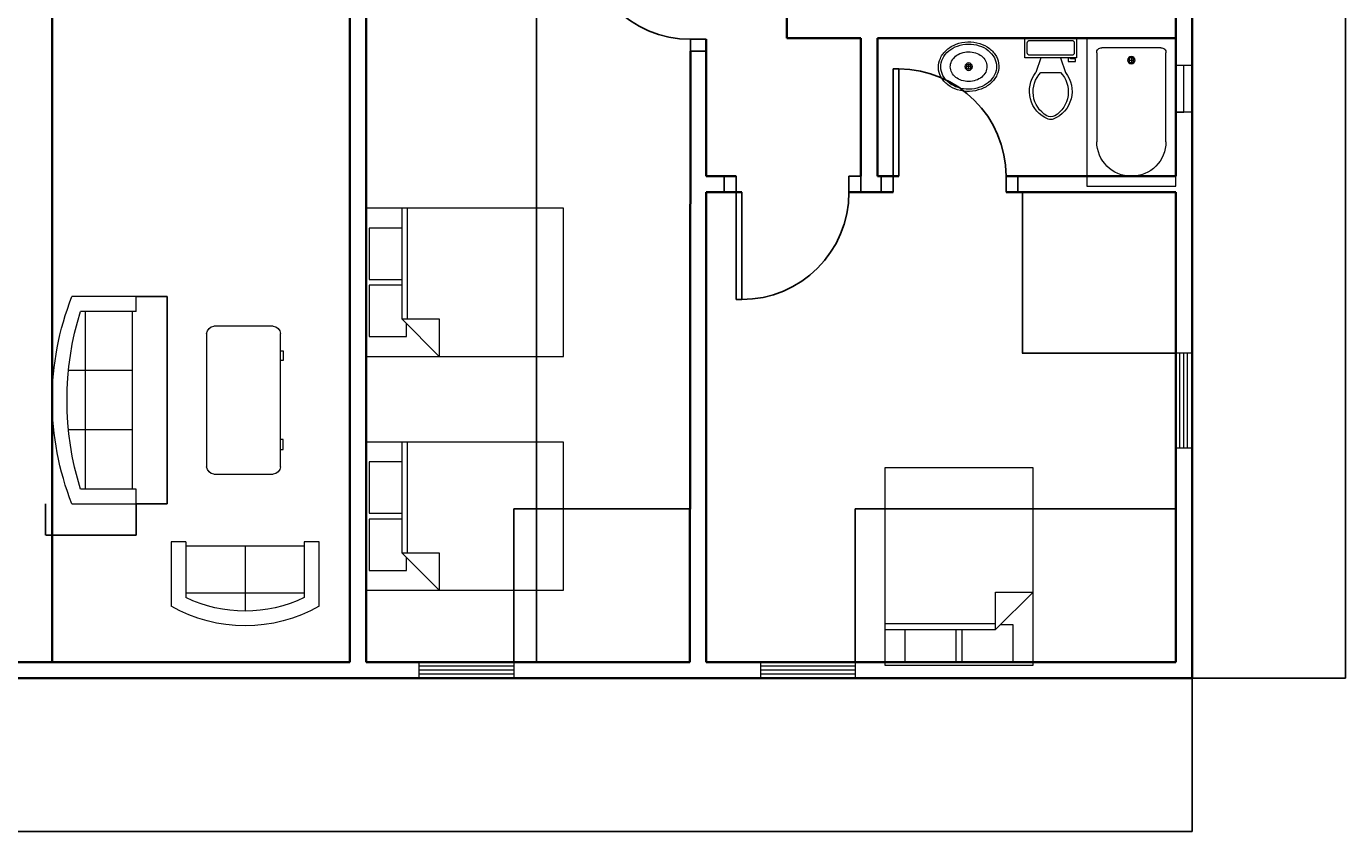
# Model space of a CAD drawing. Units: millimetres. Extents: x 31 to 27050, y -916 to 32407.
# Tile 4 of 7: x 13474 to 27050, y -916 to 7370. Entities that reach past the tile are written whole.
import ezdxf

# ---------------------------------------------------------------- set-up
doc = ezdxf.new("R2010")
doc.units = ezdxf.units.MM
for name, color, linetype, lineweight in [('A-ANNO-DIMS', 2, 'Continuous', 18), ('A-DOOR', 3, 'Continuous', 25), ('A-FLOR-FIXT', 9, 'Continuous', 18), ('A-FURN', 8, 'Continuous', 13), ('A-GLAZ', 4, 'Continuous', 18), ('A-WALL', 7, 'Continuous', 35)]:
    doc.layers.add(name, color=color, linetype=linetype, lineweight=lineweight)
doc.styles.get("Standard").update_dxf_attribs({"font": 'arial.ttf'})
doc.dimstyles.get("Standard").update_dxf_attribs({"dimtxt": 0.18, "dimasz": 0.18, "dimexe": 0.18, "dimexo": 0.0625, "dimgap": 0.09, "dimtad": 0, "dimtih": 1, "dimtoh": 1, "dimdec": 4, "dimzin": 0, "dimdsep": 46, "dimtxsty": 'Standard', "dimcen": 0.09, "dimadec": 0, "dimazin": 0, "dimtfac": 1, "dimtdec": 4, "dimtofl": 0, "dimtmove": 0, "dimatfit": 3, "dimfxl": 1, "dimtolj": 1, "dimtzin": 0, "dimarcsym": 0})

# ---------------------------------------------------------------- blocks, each defined once
blk = doc.blocks.new('Bath Tub - 26 x 60 in.')
for p, q in [((8, -18), (10, -18)), ((9, -17), (9, -19))]:
    blk.add_line(p, q)
blk.add_lwpolyline([(0, -36), (0, 0), (60, 0), (60, -36)], close=True)
for points in [[(6, -4), (42, -4)], [(4, -30), (4, -6)], [(42, -32), (6, -32)]]:
    blk.add_lwpolyline(points)
for radius in [1.5, 1]:
    blk.add_circle((9, -18), radius)
for centre, radius, start, end in [((5.75, -5.75), 1.767766999999999, 81.86989999999999, 188.1301), ((42, -18), 14, 270, 90), ((5.75, -30.25), 1.767766999999999, 171.8699, 278.1301)]:
    blk.add_arc(centre, radius, start, end)
blk = doc.blocks.new('Sink - Oval top')
for p, q in [((-1, 0), (1, 0)), ((0, 1), (0, -1))]:
    blk.add_line(p, q)
for points in [[(-12.23371880354079, 0.3941914712607968, 0.1176342565883263), (-11.46456229543957, -3.361933235489118, 0.104469279667093), (-8.878748691070427, -6.803541973650567, 0.0900157896014849), (-5.082757700676665, -9.072309807490512, 0.0819199491592185), (-0.3227280122732736, -10.01585280257211, 0.0819199491592091), (4.488169920880977, -9.380701564817912, 0.0900157896014801), (8.422342359155778, -7.36101289847943, 0.1044692796670922), (11.22435122606941, -4.093009071543406, 0.1176342565883338), (12.23371880354091, -0.3941914712607968, 0.1176342565883057), (11.46456229543992, 3.361933235488777, 0.1044692796670849), (8.878748691070427, 6.803541973650567, 0.0900157896014884), (5.082757700676324, 9.072309807490681, 0.0819199491592058), (0.3227280122732736, 10.01585280257211, 0.081919949159207), (-4.488169920880864, 9.380701564817969, 0.0900157896014802), (-8.422342359155778, 7.36101289847943, 0.1044692796670951), (-11.22435122606919, 4.093009071543633, 0.1176342565883402)], [(-11.28627986850119, 0.1590597164737346, 0.1186217001864142), (-10.51590095791209, -3.253161772358112, 0.1046781721811095), (-8.071803350560115, -6.358618019863342, 0.0895620664691738), (-4.537699193222351, -8.366971929609804, 0.0811846988912177), (-0.1289739026695997, -9.15150355811437, 0.0811846988912276), (4.300109150126218, -8.491524865184601, 0.0895620664691798), (7.889406708212618, -6.583562428127606, 0.1046781721811044), (10.42004782883111, -3.548216131892445, 0.1186217001864013), (11.28627986850119, -0.1590597164736209, 0.1186217001863945), (10.51590095791221, 3.253161772357998, 0.1046781721811069), (8.071803350560115, 6.358618019863342, 0.0895620664691756), (4.537699193222124, 8.366971929609917, 0.081184698891216), (0.1289739026695997, 9.151503558114428, 0.0811846988912142), (-4.300109150125877, 8.491524865184829, 0.0895620664691747), (-7.889406708212618, 6.583562428127606, 0.1046781721811045), (-10.42004782883111, 3.548216131892445, 0.1186217001863946)], [(-7.420452389032902, 0.0829876781601797, 0.1182825673856775), (-6.907065465214486, -2.1674649380775, 0.1046074595377274), (-5.294791470712084, -4.209988192029413, 0.0897179636260996), (-2.966599981142508, -5.528122152688069, 0.0814360825277113), (-0.0675135187855176, -6.036810076758797, 0.0814360825277218), (2.84222437824053, -5.593085960977873, 0.0897179636261315), (5.199312936802016, -4.327350491993342, 0.1046074595376878), (6.85686365682659, -2.321395784920355, 0.1182825673856714), (7.420452389033016, -0.0829876781601797, 0.1182825673856961), (6.907065465214486, 2.167464938077614, 0.1046074595377135), (5.294791470712084, 4.209988192029413, 0.0897179636261265), (2.966599981142621, 5.528122152687842, 0.0814360825277426), (0.0675135187855176, 6.036810076758797, 0.0814360825277225), (-2.842224378240644, 5.593085960977873, 0.0897179636261212), (-5.199312936802016, 4.327350491993342, 0.1046074595377049), (-6.856863656826476, 2.321395784920355, 0.1182825673856712)]]:
    blk.add_lwpolyline(points, format="xyb", close=True)
for radius in [1.5, 1]:
    blk.add_circle((0, 0), radius)
blk = doc.blocks.new('Toilet - top')
for p, q in [((9.5, -6), (9.5, -2)), ((-10, -8.5), (-8, -8.5)), ((-10, -9.5), (-10, -8.5)), ((-7, -9.5), (-10, -9.5)), ((-8, -8.5), (-8, -8)), ((-7, -8), (-7, -9.5)), ((-4, -8), (-6, -14)), ((4, -8), (6, -14)), ((4, -14), (-4, -14))]:
    blk.add_line(p, q)
blk.add_lwpolyline([(10.5, -8), (10.5, 0), (-10.5, 0), (-10.5, -8)], close=True)
for points in [[(-9.5, -2), (-9.5, -6)], [(8.5, -1), (-8.5, -1)], [(-8.5, -7), (8.5, -7)]]:
    blk.add_lwpolyline(points)
for centre, radius, start, end in [((-8.625, -1.875), 0.8838834999999999, 81.86989999999999, 188.1301), ((8.625, -1.875), 0.8838834999999999, 351.8699, 98.13009999999998), ((-8.625, -6.125), 0.8838834999999999, 171.869898, 278.1301), ((8.625, -6.125), 0.8838834999999999, 261.8699, 8.130099999999993), ((3.519562435188956, -21.58049502388982), 12.16902005083646, 141.4691096810948, 247.9714346835576), ((4.199957580658807, -21.81740929088453), 11.3291791325804, 136.3677254423718, 238.946823937405), ((-3.519499936778316, -21.58047137067522), 12.16903423757823, 292.0284332733152, 38.53070636800453), ((-4.199890672038477, -21.81738596564128), 11.32918622148567, 301.0530065773863, 43.63209216694732), ((2.09660981727e-05, -27.87646475467881), 4, 245.7318247449371, 294.2681740488959), ((2.09415214183e-05, -28.99996806116075), 4, 254.8605283244437, 285.1394707718433)]:
    blk.add_arc(centre, radius, start, end)
blk = doc.blocks.new('Sofa - Roundback 7 ft.')
for p, q in [((-12.00002, -32.44210000000393), (-12.00003, -6.597100000003898)), ((11.99996999999999, -32.44210000000393), (11.99997999999999, -6.597100000003898)), ((-36.000027, -34.00000000000395), (-36.000027, -11.46960000000396)), ((-35.999844, -13.38190000000397), (35.99979999999999, -13.38190000000397)), ((35.99997999999999, -34.00000000000395), (35.99997999999999, -11.46960000000396)), ((-36.000027, -32.44210000000393), (35.99997999999999, -32.44210000000393))]:
    blk.add_line(p, q)
for points in [[(-36.000027, -34.00000000000395), (-42.000027, -34.00000000000395), (-42.000027, -8.000000000003944)], [(41.99997999999999, -8.000000000003944), (41.99997999999999, -34.00000000000395), (35.99997999999999, -34.00000000000395)]]:
    blk.add_lwpolyline(points)
for centre, radius, start, end in [((0, -114.2500000000039), 114.2500000000039, 68.43141000000072, 111.5686000000006), ((-1.00000000032e-05, -127.1968000000039), 121.1967999999973, 72.72032999999948, 107.2797000000005)]:
    blk.add_arc(centre, radius, start, end)
blk = doc.blocks.new('Sofa - Roundback Loveseat 5 ft.')
for p, q in [((0, -32.44198000000246), (0, -5.999980000002448)), ((-23.99999999999999, -33.99998000000245), (-23.99999999999999, -11.46958000000243)), ((-23.99979999999998, -13.38178000000245), (23.99986, -13.38178000000245)), ((24.00004000000001, -33.99998000000245), (24.00004000000001, -11.46958000000243)), ((-23.99999999999999, -32.44198000000246), (24.00004000000001, -32.44198000000246))]:
    blk.add_line(p, q)
for points in [[(-23.99999999999999, -33.99998000000245), (-29.99999999999999, -33.99998000000245), (-29.99999999999999, -7.999980000002448)], [(30.00004000000001, -7.999980000002448), (30.00004000000001, -33.99998000000245), (24.00004000000001, -33.99998000000245)]]:
    blk.add_lwpolyline(points)
for centre, radius, start, end in [((0, -60.24998000000245), 60.24998000000245, 60.13715000000122, 119.862800000004), ((0, -61.38438000000245), 55.38444000000723, 64.32083000000306, 115.6791999999996)]:
    blk.add_arc(centre, radius, start, end)
blk = doc.blocks.new('Desk - 30 x 60 in.')
for p, q in [((-26.999995, 0), (26.999995, 0)), ((-29.999995, -27), (-29.999995, -3)), ((29.999995, -3), (29.999995, -27)), ((26.999995, -30), (-26.999995, -30)), ((-20.000005, -30), (-20.000005, -31)), ((-20.000005, -31), (-16.000005, -31)), ((-16.000005, -31), (-16.000005, -30)), ((15.999995, -31), (15.999995, -30)), ((19.999995, -31), (15.999995, -31)), ((19.999995, -30), (19.999995, -31))]:
    blk.add_line(p, q)
for centre, radius, start, end in [((-26.499995, -3.5), 3.535534000004229, 98.1300999999916, 171.8698999999352), ((26.499995, -3.5), 3.535533999997753, 8.130102000022115, 81.8698999999439), ((-26.499995, -26.5), 3.535534000000845, 188.1301000000653, 261.8699000000085), ((26.499995, -26.5), 3.535534000004826, 278.1301000000561, 351.8698999999439)]:
    blk.add_arc(centre, radius, start, end)
blk = doc.blocks.new('Bed - Queen')
for p, q in [((0, -80.00003000000002), (0, 0)), ((0, 0), (59.99998999999999, 0)), ((59.99998999999999, 0), (59.99998999999999, -80.00003000000002)), ((7.99999, -1.200000000000017), (28.79998, -1.200000000000017)), ((7.99999, -14.4), (7.99999, -1.200000000000017)), ((28.79998, -1.200000000000017), (28.79998, -14.4)), ((31.19999, -1.200000000000017), (51.99999000000001, -1.200000000000017)), ((31.19999, -14.4), (31.19999, -1.200000000000017)), ((51.99999000000001, -1.200000000000017), (51.99999000000001, -16.4)), ((0, -14.4), (44.79999999999999, -14.4)), ((59.99998999999999, -29.60000000000001), (44.79999999999999, -14.4)), ((44.79999999999999, -14.4), (44.79999999999999, -29.60000000000001)), ((44.79999999999999, -16.80000000000001), (0, -16.80000000000001)), ((51.99999000000001, -16.4), (46.79936, -16.4)), ((44.79999999999999, -29.60000000000001), (59.99998999999999, -29.60000000000001)), ((59.99998999999999, -80.00003000000002), (0, -80.00003000000002))]:
    blk.add_line(p, q)
blk = doc.blocks.new('Window - Wood Frame 36 in. Wide plan')
for p, q in [((0, 6), (0, 0)), ((36, 6), (36, 0)), ((0, 4.5), (36, 4.5)), ((0, 3), (36, 3)), ((0, 1.5), (36, 1.5))]:
    blk.add_line(p, q)
blk = doc.blocks.new('DOOR-SINGLE-1104')
for p, q in [((56.41678681898429, 1104.337341461596), (-7.18501e-11, 1104.337341461596)), ((-7.18501e-11, 1104.337341461596), (-7.18501e-11, 3.638e-12)), ((56.41678681898429, 7.276e-12), (56.41678681898429, 1104.337341461596)), ((-1226.913698425656, -163.8831223050438), (-1226.913698425656, 3.638e-12)), ((-1104.337341461589, 3.638e-12), (-1226.913698425656, 7.276e-12)), ((-1104.337341461589, 3.638e-12), (-1104.337341461589, -163.8831223050438)), ((-7.18501e-11, 3.638e-12), (56.41678681898429, 7.276e-12)), ((56.41678681898429, -163.8831223050438), (56.41678681898429, 3.638e-12)), ((56.41678681898429, 3.638e-12), (178.9931437830519, 3.638e-12)), ((178.9931437830519, 3.638e-12), (178.9931437830519, -163.8831223050438)), ((-1104.337341461589, -163.8831223050438), (-1226.913698425656, -163.8831223050438)), ((178.9931437830519, -163.8831223050438), (56.41678681898429, -163.8831223050438))]:
    blk.add_line(p, q)
blk.add_arc((0, 3.638e-12), 1104.337341461589, 90, 180)
blk = doc.blocks.new('WIN-BATH-482-FRAMED')
for p, q in [((-2.274e-13, -9.095e-13), (-168.3506507106942, -9.095e-13)), ((-168.3506507106942, -9.095e-13), (-168.3506507106942, -482.3297634273203)), ((-84.17532535534656, -482.3297634273203), (-84.17532535534723, -9.095e-13)), ((-168.3506507106942, -482.3297634273203), (1.1369e-12, -482.3297634273195)), ((1.1369e-12, -482.3297634273195), (-84.17532535534656, -482.3297634273203))]:
    blk.add_line(p, q)
blk = doc.blocks.new('*D34')
at = {"layer": 'A-ANNO-DIMS', "color": 0, "lineweight": -2, "transparency": 16777216}
for p, q in [((14604.24783261055, 4589.760747355135), (14924.40539496012, 4589.760747355135)), ((14924.22539496012, 4589.580747355134), (14924.22539496012, 3523.143731883442)), ((14924.22539496012, 2456.340331691422), (14924.22539496012, 3522.777347163115)), ((14604.24783261055, 2456.160331691423), (14924.40539496012, 2456.160331691423))]:
    blk.add_line(p, q, dxfattribs=at)
at = {"layer": 'A-ANNO-DIMS', "color": 0, "transparency": 16777216}
for points in [[(14924.19539496012, 4589.580747355134), (14924.25539496012, 4589.580747355134), (14924.22539496012, 4589.760747355135)], [(14924.19539496012, 2456.340331691422), (14924.25539496012, 2456.340331691422), (14924.22539496012, 2456.160331691423)]]:
    blk.add_solid(points, dxfattribs=at)
at = {"layer": 'Defpoints', "color": 0, "transparency": 16777216}
for p in [(14604.18533261055, 4589.760747355135), (14604.18533261055, 2456.160331691423), (14924.22539496012, 2456.160331691423)]:
    blk.add_point(p, dxfattribs=at)
at = {"layer": 'A-ANNO-DIMS', "color": 0, "transparency": 16777216, "insert": (14924.22539496011, 3522.960539523273), "char_height": 0.18, "attachment_point": 5}
blk.add_mtext('\\A1;SOFA 2134 TYP.', dxfattribs=at)
blk = doc.blocks.new('*D35')
at = {"layer": 'A-ANNO-DIMS', "color": 0, "lineweight": -2, "transparency": 16777216}
for p, q in [((13672.85197055589, 2456.097831691422), (13672.85197055589, 2135.940269341865)), ((14604.18533261055, 2456.097831691422), (14604.18533261055, 2135.940269341865)), ((13673.03197055589, 2136.120269341865), (14137.9206365764, 2136.120269341865)), ((14604.00533261055, 2136.120269341865), (14139.11666659004, 2136.120269341865))]:
    blk.add_line(p, q, dxfattribs=at)
at = {"layer": 'A-ANNO-DIMS', "color": 0, "transparency": 16777216}
for points in [[(13673.03197055589, 2136.150269341865), (13673.03197055589, 2136.090269341865), (13672.85197055589, 2136.120269341865)], [(14604.00533261055, 2136.150269341865), (14604.00533261055, 2136.090269341865), (14604.18533261055, 2136.120269341865)]]:
    blk.add_solid(points, dxfattribs=at)
at = {"layer": 'Defpoints', "color": 0, "transparency": 16777216}
for p in [(13672.85197055589, 2456.160331691422), (14604.18533261055, 2456.160331691422), (13672.85197055589, 2136.120269341865)]:
    blk.add_point(p, dxfattribs=at)
at = {"layer": 'A-ANNO-DIMS', "color": 0, "transparency": 16777216, "insert": (14138.51865158322, 2136.120269341865), "char_height": 0.18, "attachment_point": 5}
blk.add_mtext('\\A1;931 TYP.', dxfattribs=at)
blk = doc.blocks.new('*D46')
at = {"layer": 'A-ANNO-DIMS', "color": 0, "lineweight": -2, "transparency": 16777216}
for p, q in [((1610.021997, 663.585636), (1610.021997, -915.531864)), ((25471.148668, 663.585636), (25471.148668, -915.531864)), ((1610.201997, -915.3518639999999), (13540.17247438267, -915.3518639999999)), ((25470.968668, -915.3518639999999), (13540.99819061733, -915.3518639999999))]:
    blk.add_line(p, q, dxfattribs=at)
at = {"layer": 'A-ANNO-DIMS', "color": 0, "transparency": 16777216}
for points in [[(1610.201997, -915.321864), (1610.201997, -915.381864), (1610.021997, -915.3518639999999)], [(25470.968668, -915.321864), (25470.968668, -915.381864), (25471.148668, -915.3518639999999)]]:
    blk.add_solid(points, dxfattribs=at)
at = {"layer": 'Defpoints', "color": 0, "transparency": 16777216}
for p in [(1610.021997, 663.648136), (25471.148668, 663.648136), (25471.148668, -915.3518639999999)]:
    blk.add_point(p, dxfattribs=at)
at = {"layer": 'A-ANNO-DIMS', "color": 0, "transparency": 16777216, "insert": (13540.5853325, -915.3518639999999), "char_height": 0.18, "attachment_point": 5}
blk.add_mtext('\\A1;23861', dxfattribs=at)
blk = doc.blocks.new('*D47')
at = {"layer": 'A-ANNO-DIMS', "color": 0, "lineweight": -2, "transparency": 16777216}
for p, q in [((25471.21116800002, 30827.53125900001), (27050.32866800003, 30827.53125900001)), ((27050.14866800003, 30827.35125900001), (27050.14866800003, 15745.77166202933)), ((27050.14866800004, 663.8281360000004), (27050.14866800003, 15745.40773297067)), ((25471.21116800002, 663.6481360000002), (27050.32866800003, 663.6481360000004))]:
    blk.add_line(p, q, dxfattribs=at)
at = {"layer": 'A-ANNO-DIMS', "color": 0, "transparency": 16777216}
for points in [[(27050.11866800003, 30827.35125900001), (27050.17866800003, 30827.35125900001), (27050.14866800003, 30827.53125900001)], [(27050.11866800004, 663.8281360000004), (27050.17866800004, 663.8281360000004), (27050.14866800004, 663.6481360000004)]]:
    blk.add_solid(points, dxfattribs=at)
at = {"layer": 'Defpoints', "color": 0, "transparency": 16777216}
for p in [(25471.14866800002, 30827.53125900001), (27050.14866800003, 30827.53125900001), (25471.14866800002, 663.6481360000002)]:
    blk.add_point(p, dxfattribs=at)
at = {"layer": 'A-ANNO-DIMS', "color": 0, "transparency": 16777216, "insert": (27050.14866800003, 15745.58969749999), "char_height": 0.18, "attachment_point": 5}
blk.add_mtext('\\A1;30164', dxfattribs=at)
blk = doc.blocks.new('*D65')
at = {"layer": 'A-ANNO-DIMS', "color": 0, "lineweight": -2, "transparency": 16777216}
for p, q in [((20302.73551700001, 8571.211099000004), (18723.61801700001, 8571.211099000004)), ((18723.79801700001, 8571.031099000003), (18723.79801700001, 4699.551179000002)), ((18723.79801700001, 827.7112590000002), (18723.79801700001, 4699.191179000002)), ((20302.73551700001, 827.5312590000003), (18723.61801700001, 827.5312590000002))]:
    blk.add_line(p, q, dxfattribs=at)
at = {"layer": 'A-ANNO-DIMS', "color": 0, "transparency": 16777216}
for points in [[(18723.76801700001, 8571.031099000003), (18723.82801700001, 8571.031099000003), (18723.79801700001, 8571.211099000004)], [(18723.76801700001, 827.7112590000002), (18723.82801700001, 827.7112590000002), (18723.79801700001, 827.5312590000002)]]:
    blk.add_solid(points, dxfattribs=at)
at = {"layer": 'Defpoints', "color": 0, "transparency": 16777216}
for p in [(18723.79801700001, 8571.211099000004), (20302.79801700001, 8571.211099000004), (20302.79801700001, 827.5312590000003)]:
    blk.add_point(p, dxfattribs=at)
at = {"layer": 'A-ANNO-DIMS', "color": 0, "transparency": 16777216, "insert": (18723.79801700001, 4699.371178999996), "char_height": 0.18, "attachment_point": 5}
blk.add_mtext('\\A1;7744', dxfattribs=at)
blk = doc.blocks.new('*D78')
at = {"layer": 'A-ANNO-DIMS', "color": 0, "lineweight": -2, "transparency": 16777216}
for p, q in [((22004.509337, 827.5937589999999), (22004.509337, 2406.711259)), ((22004.689337, 2406.531259), (23653.29478204775, 2406.531259)), ((25302.618017, 2406.531259), (23654.01257195225, 2406.531259)), ((25302.798017, 827.5937589999999), (25302.798017, 2406.711259))]:
    blk.add_line(p, q, dxfattribs=at)
at = {"layer": 'A-ANNO-DIMS', "color": 0, "transparency": 16777216}
for points in [[(22004.689337, 2406.561259), (22004.689337, 2406.501259), (22004.509337, 2406.531259)], [(25302.618017, 2406.561259), (25302.618017, 2406.501259), (25302.798017, 2406.531259)]]:
    blk.add_solid(points, dxfattribs=at)
at = {"layer": 'Defpoints', "color": 0, "transparency": 16777216}
for p in [(25302.798017, 2406.531259), (22004.509337, 827.531259), (25302.798017, 827.531259)]:
    blk.add_point(p, dxfattribs=at)
at = {"layer": 'A-ANNO-DIMS', "color": 0, "transparency": 16777216, "insert": (23653.653677, 2406.531259), "char_height": 0.18, "attachment_point": 5}
blk.add_mtext('\\A1;3298', dxfattribs=at)
blk = doc.blocks.new('*D79')
at = {"layer": 'A-ANNO-DIMS', "color": 0, "lineweight": -2, "transparency": 16777216}
for p, q in [((18490.755325, 827.5937589999999), (18490.755325, 2406.711259)), ((18490.935325, 2406.531259), (19396.4272917367, 2406.531259)), ((20302.618017, 2406.531259), (19397.1260502633, 2406.531259)), ((20302.798017, 827.5937589999999), (20302.798017, 2406.711259))]:
    blk.add_line(p, q, dxfattribs=at)
at = {"layer": 'A-ANNO-DIMS', "color": 0, "transparency": 16777216}
for points in [[(18490.935325, 2406.561259), (18490.935325, 2406.501259), (18490.755325, 2406.531259)], [(20302.618017, 2406.561259), (20302.618017, 2406.501259), (20302.798017, 2406.531259)]]:
    blk.add_solid(points, dxfattribs=at)
at = {"layer": 'Defpoints', "color": 0, "transparency": 16777216}
for p in [(20302.798017, 2406.531259), (18490.755325, 827.531259), (20302.798017, 827.531259)]:
    blk.add_point(p, dxfattribs=at)
at = {"layer": 'A-ANNO-DIMS', "color": 0, "transparency": 16777216, "insert": (19396.776671, 2406.531259), "char_height": 0.18, "attachment_point": 5}
blk.add_mtext('\\A1;1812', dxfattribs=at)
blk = doc.blocks.new('*D83')
at = {"layer": 'A-ANNO-DIMS', "color": 0, "lineweight": -2, "transparency": 16777216}
for p, q in [((25302.73551700001, 5663.648136000002), (23723.61801700002, 5663.648136000002)), ((23723.79801700001, 5663.468136000002), (23723.79801700001, 4835.129304637792)), ((23723.79801700001, 4006.426667000002), (23723.79801700001, 4834.765498362211)), ((25302.73551700001, 4006.246667000001), (23723.61801700002, 4006.246667000001))]:
    blk.add_line(p, q, dxfattribs=at)
at = {"layer": 'A-ANNO-DIMS', "color": 0, "transparency": 16777216}
for points in [[(23723.76801700002, 5663.468136000002), (23723.82801700001, 5663.468136000002), (23723.79801700001, 5663.648136000002)], [(23723.76801700002, 4006.426667000002), (23723.82801700001, 4006.426667000002), (23723.79801700001, 4006.246667000001)]]:
    blk.add_solid(points, dxfattribs=at)
at = {"layer": 'Defpoints', "color": 0, "transparency": 16777216}
for p in [(23723.79801700001, 5663.648136000002), (25302.79801700002, 5663.648136000002), (25302.79801700002, 4006.246667000001)]:
    blk.add_point(p, dxfattribs=at)
at = {"layer": 'A-ANNO-DIMS', "color": 0, "transparency": 16777216, "insert": (23723.79801700001, 4834.947401499993), "char_height": 0.18, "attachment_point": 5}
blk.add_mtext('\\A1;1657.4', dxfattribs=at)

msp = doc.modelspace()

# ---------------------------------------------------------------- linework, layer by layer
at = {"layer": 'A-DOOR'}
for p, q in [((20656.40295751389, 5663.648136366686), (20656.40295751389, 5827.531258671734)), ((22061.20428885169, 5827.531258671735), (21939.73344275853, 5827.531258671735))]:
    msp.add_line(p, q, dxfattribs=at)
at = {"layer": 'A-WALL'}
for p, q in [((13740.58533261045, 827.5312586717337), (13740.58533261045, 12938.12750679554)), ((16802.79801739574, 12938.12750679554), (16802.79801739574, 827.5312586717337)), ((25471.14866810643, 744.3803777755929), (25471.14866810643, 12465.74367114627)), ((25302.79801739574, 5827.531258671735), (25302.79801739574, 12301.86054884122)), ((16971.14866810643, 8571.211098631777), (16971.14866810643, 827.5312586717337)), ((21299.46298919959, 8679.383477017574), (21299.46298919959, 7331.275946538546)), ((21299.46298919959, 7250.543705129635), (21299.46298919959, 7331.275946538546)), ((20471.14866810643, 5827.531258671733), (20471.14866810643, 7237.845399735471)), ((21387.2503044143, 7250.543705129635), (21299.46298919959, 7250.543705129635)), ((21387.2503044143, 7250.543705129635), (22061.20428885169, 7250.543705129635)), ((22061.20428885169, 7250.543705129635), (22061.20428885169, 5827.531258671735)), ((22234.39825211639, 7250.543705129635), (22234.39825211639, 5827.531258671734)), ((22234.39825211639, 7250.543705129635), (25302.79801739574, 7250.543705129636)), ((20307.26554580138, 7115.269042771405), (20302.79801739574, 827.5312586717337)), ((20778.97931447796, 5827.531258671733), (20471.14866810643, 5827.531258671733)), ((22451.48878877845, 5827.531258671734), (22234.39825211639, 5827.531258671734)), ((25302.79801739574, 5827.531258671735), (23555.82613023996, 5827.531258671734)), ((20835.39610129702, 5663.648136366682), (20471.14866810643, 5663.648136366682)), ((20471.14866810643, 827.5312586717337), (20471.14866810643, 5663.648136366681)), ((22395.07200195939, 5663.648136366682), (21939.73344275853, 5663.648136366682)), ((25302.79801739574, 5663.648136366682), (23555.82613023996, 5663.648136366682)), ((25302.79801739574, 827.5312586717337), (25302.79801739574, 5663.648136366682)), ((13540.58533261045, 827.5312586717337), (10390.58533261045, 827.5312586717337)), ((13540.58533261045, 827.5312586717337), (16690.58533261045, 827.5312586717337)), ((16802.79801739574, 827.5312586717337), (13740.58533261045, 827.5312586717336)), ((20302.79801739574, 827.5312586717337), (16971.14866810643, 827.5312586717337)), ((25302.79801739574, 827.5312586717337), (20471.14866810643, 827.5312586717337)), ((25471.14866810643, 744.3803777755929), (25471.14866810643, 663.6481363666826)), ((10190.58533261045, 663.6481363666826), (16690.58533261045, 663.6481363666826)), ((16890.58533261045, 663.6481363666826), (10390.58533261045, 663.6481363666826)), ((25390.58533261046, 663.6481363666826), (16890.58533261045, 663.6481363666826)), ((25471.14866810643, 663.6481363666826), (25390.58533261046, 663.6481363666826))]:
    msp.add_line(p, q, dxfattribs=at)

# ---------------------------------------------------------------- block references
at = {"layer": 'A-DOOR'}
for p, rotation in [((20307.26554580139, 8342.182741197055), 89.99999999999982), ((20835.39610129696, 5663.648136366701), 180)]:
    msp.add_blockref('DOOR-SINGLE-1104', p, dxfattribs=dict(at, rotation=rotation))
at = {"layer": 'A-DOOR', "extrusion": (0, 0, -1), "zscale": -1}
msp.add_blockref('DOOR-SINGLE-1104', (-22451.48878877838, 5827.531258671719), dxfattribs=at)
at = {"layer": 'A-FLOR-FIXT', "xscale": -25.4, "yscale": 25.4, "zscale": 25.4}
for name, p in [('Sink - Oval top', (23171.10041040371, 6955.654409605282)), ('Toilet - top', (24015.84997535291, 7250.543705129635))]:
    msp.add_blockref(name, p, dxfattribs=at)
at = {"layer": 'A-FLOR-FIXT', "xscale": -25.4, "yscale": 25.4, "zscale": 25.4, "rotation": 90}
msp.add_blockref('Bath Tub - 26 x 60 in.', (24388.39801739574, 7250.543705129635), dxfattribs=at)
at = {"layer": 'A-FURN', "xscale": -25.4, "yscale": 25.4, "zscale": 25.4}
for name, p, rotation in [('Bed - Queen', (16971.14866810643, 5498.496041437785), 90), ('Sofa - Roundback 7 ft.', (13740.58533261045, 3522.960061555132), 90), ('Desk - 30 x 60 in.', (15328.78238791416, 3524.348674154725), 90), ('Bed - Queen', (16971.14866810643, 3091.368000807226), 90), ('Bed - Queen', (22309.86417738938, 797.0512586717331), 180), ('Sofa - Roundback Loveseat 5 ft.', (15725.13818008764, 1201.42641839608), 180)]:
    msp.add_blockref(name, p, dxfattribs=dict(at, rotation=rotation))
at = {"layer": 'A-GLAZ', "extrusion": (0, 0, -1), "zscale": -1}
msp.add_blockref('WIN-BATH-482-FRAMED', (-25302.79801739574, 6971.117434470521), dxfattribs=at)
at = {"layer": 'A-GLAZ', "xscale": -27.11229900122799, "yscale": 27.11229900122799, "zscale": 27.11229900122799, "rotation": 270}
msp.add_blockref('Window - Wood Frame 36 in. Wide plan', (25302.79801739574, 3030.203903365821), dxfattribs=at)
at = {"layer": 'A-GLAZ', "xscale": -27.11229900122799, "yscale": 27.11229900122799, "zscale": 27.11229900122799}
for p in [(18490.75532509744, 664.8574646643647), (22004.50933705546, 664.8574646643647)]:
    msp.add_blockref('Window - Wood Frame 36 in. Wide plan', p, dxfattribs=at)

# ---------------------------------------------------------------- dimensions: what is measured, and where the dimension line sits
at = {"layer": 'A-ANNO-DIMS'}
for base, p1, p2, angle, override, picture, middle in [((27050.14866800003, 30827.53125900001), (25471.148668, 663.648136), (25471.148668, 30827.531259), 90, {"dimdec": 0, "dimlfac": 1, "dimrnd": 0, "dimzin": 0, "dimdsep": 46, "dimlunit": 2}, '*D47', (27050.14866800003, 15745.58969749999)), ((18723.79801700001, 8571.211099000004), (20302.798017, 827.531259), (20302.798017, 8571.211099), 90, {"dimdec": 0, "dimlfac": 1, "dimrnd": 0, "dimzin": 0, "dimdsep": 46, "dimlunit": 2}, '*D65', (18723.79801700001, 4699.371178999996)), ((23723.79801700001, 5663.648136000002), (25302.798017, 4006.246667), (25302.798017, 5663.648135999999), 90, {"dimdec": 1, "dimlfac": 1, "dimrnd": 0, "dimzin": 0, "dimdsep": 46, "dimlunit": 2}, '*D83', (23723.79801700001, 4834.947401499993)), ((20302.798017, 2406.531259), (18490.755325, 827.531259), (20302.798017, 827.531259), 3.59e-14, {"dimdec": 0, "dimlfac": 1, "dimrnd": 0, "dimzin": 0, "dimdsep": 46, "dimlunit": 2}, '*D79', (19396.776671, 2406.531259)), ((25302.798017, 2406.531259), (22004.509337, 827.531259), (25302.798017, 827.531259), 1.97e-14, {"dimdec": 0, "dimlfac": 1, "dimrnd": 0, "dimzin": 0, "dimdsep": 46, "dimlunit": 2}, '*D78', (23653.653677, 2406.531259))]:
    dim = msp.add_linear_dim(base=base, p1=p1, p2=p2, angle=angle, dimstyle='Standard', override=override, dxfattribs=at)
    dim.commit()
    dim.dimension.update_dxf_attribs({"geometry": picture, "text_midpoint": middle})
for base, p1, p2, angle, text, picture, middle in [((14924.22539496012, 2456.160331691423), (14604.18533261055, 4589.760747355132), (14604.18533261055, 2456.160331691422), 270, 'SOFA <> TYP.', '*D34', (14924.22539496011, 3522.960539523273)), ((13672.85197055589, 2136.120269341865), (14604.18533261055, 2456.160331691422), (13672.85197055589, 2456.160331691422), 180, '<> TYP.', '*D35', (14138.51865158322, 2136.120269341865))]:
    dim = msp.add_linear_dim(base=base, p1=p1, p2=p2, angle=angle, text=text, dimstyle='Standard', override={"dimdec": 0, "dimlfac": 1, "dimrnd": 0, "dimzin": 0, "dimdsep": 46, "dimlunit": 2}, dxfattribs=at)
    dim.commit()
    dim.dimension.update_dxf_attribs({"geometry": picture, "text_midpoint": middle})
dim = msp.add_linear_dim(base=(25471.148668, -915.3518639999999), p1=(1610.021997, 663.648136), p2=(25471.148668, 663.648136), dimstyle='Standard', override={"dimdec": 0, "dimlfac": 1, "dimrnd": 0, "dimzin": 0, "dimdsep": 46, "dimlunit": 2}, dxfattribs=at)
dim.commit()
dim.dimension.update_dxf_attribs({"geometry": '*D46', "text_midpoint": (13540.5853325, -915.3518639999999)})

doc.saveas('drawing.dxf')
